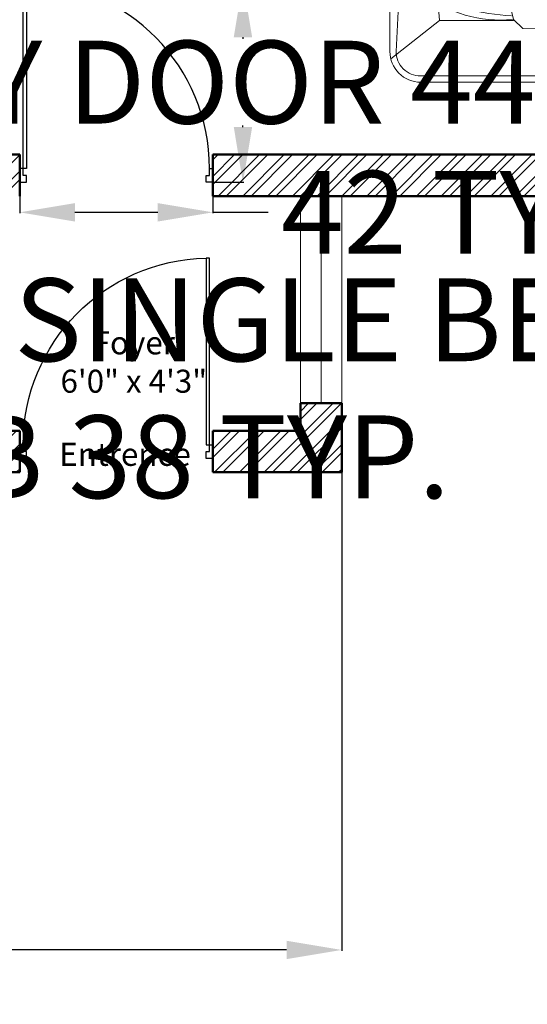
# Model space of a CAD drawing. Units: inches. Extents: x -90 to 536, y -553 to 299.
# Tile 10 of 27: x 191 to 301, y -553 to -339. Entities that reach past the tile are written whole.
import ezdxf

# ---------------------------------------------------------------- set-up
doc = ezdxf.new("R2010")
doc.units = ezdxf.units.IN
for name, color, linetype, lineweight in [('A-ANNO-DIMS', 2, 'Continuous', 18), ('A-ANNO-TEXT', 7, 'Continuous', 18), ('A-AREA-IDEN', 7, 'Continuous', 18), ('A-DOOR', 4, 'Continuous', 25), ('A-GLAZ', 4, 'Continuous', 18), ('A-WALL-PATT', 252, 'Continuous', 13), ('Furniture', 2, 'Continuous', 18), ('Outer Wall', 1, 'Continuous', 50)]:
    doc.layers.add(name, color=color, linetype=linetype, lineweight=lineweight)
doc.styles.get("Standard").update_dxf_attribs({"font": 'arial.ttf'})
doc.dimstyles.get("Standard").update_dxf_attribs({"dimtxt": 18, "dimasz": 12, "dimexe": 0.18, "dimexo": 0.0625, "dimgap": 0.09, "dimtad": 0, "dimtih": 1, "dimtoh": 1, "dimdec": 0, "dimzin": 0, "dimdsep": 46, "dimlunit": 3, "dimtxsty": 'Standard', "dimcen": 0.09, "dimadec": 0, "dimazin": 0, "dimtfac": 1, "dimtdec": 0, "dimtofl": 0, "dimtmove": 0, "dimatfit": 3, "dimfxl": 1, "dimtolj": 1, "dimtzin": 0, "dimarcsym": 0})

# ---------------------------------------------------------------- blocks, each defined once
blk = doc.blocks.new('A$C4DC51D13')
for p, q in [((3265.3, 2996.2), (1188.4, 2996.2)), ((1895.2, 2134), (1895.2, 2996.2)), ((2559.6, 2996.2), (2559.6, 2617.8)), ((277.4, 2939.6), (277.4, 2141.8)), ((943, 2103.5), (943, 2936.7)), ((1188.4, 2962.7), (1862.1, 2962.7)), ((1862.1, 2134), (1862.1, 2962.7)), ((1928.3, 2961.6), (2524.2, 2961.6)), ((1928.3, 2134), (1928.3, 2961.6)), ((2524.2, 2961.6), (2524.2, 2658.6)), ((2590.4, 2962.7), (2590.4, 2654.5)), ((3265.3, 2962.7), (2590.4, 2962.7)), ((1018.2, 2892.3), (232.2, 2892.3)), ((304, 2865.7), (304, 2253.3)), ((916.4, 2865.7), (304, 2865.7)), ((916.4, 2253.3), (916.4, 2865.7)), ((1290.4, 2664.8), (1028, 2870.9)), ((3163.3, 2664.8), (3425.7, 2870.9)), ((3778.5, 2897), (3631.2, 2747.3)), ((4008.9, 2375.5), (3778.5, 2897)), ((4156.2, 2525.2), (3778.5, 2897)), ((1022.9, 2163.8), (1022.9, 2830.3)), ((1056, 2830.3), (1081, 2194.8)), ((3397.7, 2830.3), (3364.5, 2194.8)), ((3430.8, 2163.8), (3430.8, 2830.3)), ((423.7, 2370.8), (776.6, 2723.7)), ((427.4, 2727.4), (772.8, 2367.1)), ((506.4, 2652.2), (506.4, 2704.4)), ((510.6, 2655.8), (510.6, 2706.9)), ((514.9, 2659.2), (514.9, 2709.2)), ((519.1, 2662.3), (519.1, 2711.3)), ((523.3, 2665.1), (523.3, 2713.4)), ((527.5, 2667.8), (527.5, 2715.2)), ((531.8, 2670.2), (531.8, 2717)), ((536, 2672.5), (536, 2718.7)), ((540.2, 2674.6), (540.2, 2720.2)), ((544.4, 2676.5), (544.4, 2721.6)), ((548.7, 2678.2), (548.7, 2722.9)), ((650.1, 2678.8), (650.1, 2723.3)), ((654.3, 2677.1), (654.3, 2722)), ((658.6, 2675.2), (658.6, 2720.7)), ((662.8, 2673.2), (662.8, 2719.2)), ((667, 2671), (667, 2717.6)), ((668.5, 2670.2), (668.5, 2717)), ((671.2, 2668.6), (671.2, 2715.9)), ((672.7, 2667.8), (672.7, 2715.2)), ((675.5, 2666.1), (675.5, 2714)), ((676.9, 2665.1), (676.9, 2713.4)), ((679.7, 2663.3), (679.7, 2712)), ((681.1, 2662.3), (681.1, 2711.3)), ((683.9, 2660.3), (683.9, 2709.9)), ((685.4, 2659.2), (685.4, 2709.2)), ((688.1, 2657), (688.1, 2707.7)), ((689.6, 2655.8), (689.6, 2706.9)), ((692.4, 2653.5), (692.4, 2705.3)), ((693.8, 2652.2), (693.8, 2704.4)), ((4008.9, 2375.5), (3631.2, 2747.3)), ((448.9, 2650.4), (504.4, 2650.4)), ((451.5, 2440.6), (451.5, 2654)), ((451.9, 2654.6), (509.2, 2654.6)), ((455.1, 2658.8), (514.4, 2658.8)), ((455.7, 2434.9), (455.7, 2659.6)), ((458.4, 2663.1), (520.2, 2663.1)), ((459.9, 2558.8), (459.9, 2664.9)), ((462, 2667.3), (526.7, 2667.3)), ((464.1, 2583.3), (464.1, 2669.7)), ((465.8, 2671.5), (534.1, 2671.5)), ((468.4, 2596.6), (468.4, 2674.3)), ((469.8, 2675.7), (542.8, 2675.7)), ((472.6, 2606.7), (472.6, 2678.5)), ((476.8, 2615), (476.8, 2682.5)), ((481, 2622.2), (481, 2686.2)), ((485.3, 2628.5), (485.3, 2689.7)), ((489.5, 2634.2), (489.5, 2693)), ((489.5, 2667.3), (489.5, 2633.5)), ((493.7, 2639.3), (493.7, 2696.1)), ((497.9, 2644), (497.9, 2699.1)), ((502.2, 2648.3), (502.2, 2701.8)), ((657.4, 2675.7), (730.4, 2675.7)), ((734.5, 2671.5), (666.1, 2671.5)), ((666.1, 2671.5), (734.5, 2671.5)), ((738.2, 2667.3), (673.5, 2667.3)), ((673.5, 2667.3), (738.2, 2667.3)), ((741.8, 2663.1), (680, 2663.1)), ((680, 2663.1), (741.8, 2663.1)), ((745.2, 2658.8), (685.8, 2658.8)), ((685.8, 2658.8), (745.2, 2658.8)), ((748.3, 2654.6), (691, 2654.6)), ((691, 2654.6), (748.3, 2654.6)), ((751.3, 2650.4), (695.8, 2650.4)), ((695.8, 2650.4), (751.3, 2650.4)), ((696.6, 2649.6), (696.6, 2702.7)), ((698, 2648.3), (698, 2701.8)), ((700.8, 2645.5), (700.8, 2700)), ((702.3, 2644), (702.3, 2699.1)), ((705, 2641), (705, 2697.2)), ((706.5, 2639.3), (706.5, 2696.1)), ((709.3, 2636), (709.3, 2694.1)), ((710.7, 2634.2), (710.7, 2693)), ((713.5, 2630.5), (713.5, 2690.9)), ((714.9, 2628.5), (714.9, 2689.7)), ((717.7, 2624.4), (717.7, 2687.4)), ((719.2, 2622.2), (719.2, 2686.2)), ((722, 2617.6), (722, 2683.8)), ((723.4, 2615), (723.4, 2682.5)), ((726.2, 2609.7), (726.2, 2679.9)), ((727.6, 2606.7), (727.6, 2678.5)), ((730.4, 2600.3), (730.4, 2675.7)), ((731.9, 2596.6), (731.9, 2674.3)), ((734.6, 2588.4), (734.6, 2671.3)), ((736.1, 2583.3), (736.1, 2669.7)), ((738.9, 2570.4), (738.9, 2666.6)), ((740.3, 2558.8), (740.3, 2664.9)), ((743.1, 2433.1), (743.1, 2661.5)), ((744.5, 2434.9), (744.5, 2659.6)), ((747.3, 2438.6), (747.3, 2656)), ((748.8, 2440.6), (748.8, 2654)), ((1283.3, 2574.2), (1290.4, 2664.8)), ((1290.4, 2664.8), (1894.7, 2664.8)), ((1895.2, 2663.7), (2557.3, 2663.7)), ((2603.6, 2664.8), (2559, 2664.8)), ((3163.3, 2664.8), (2764.7, 2664.8)), ((3170.4, 2574.2), (3163.3, 2664.8)), ((3631.7, 2676.6), (3938.2, 2375)), ((424.8, 2599.7), (469.6, 2599.7)), ((426.1, 2603.9), (471.3, 2603.9)), ((426.1, 2490.7), (426.1, 2603.9)), ((427.5, 2608.1), (473.3, 2608.1)), ((429.1, 2612.3), (475.4, 2612.3)), ((430.3, 2479), (430.3, 2615.5)), ((430.7, 2616.6), (477.7, 2616.6)), ((432.5, 2620.8), (480.2, 2620.8)), ((434.5, 2469.3), (434.5, 2625.2)), ((434.5, 2625), (482.9, 2625)), ((436.5, 2629.2), (485.8, 2629.2)), ((438.7, 2633.5), (488.9, 2633.5)), ((438.8, 2460.9), (438.8, 2633.6)), ((441, 2637.7), (492.3, 2637.7)), ((443, 2453.4), (443, 2641.1)), ((443.5, 2641.9), (496, 2641.9)), ((446.1, 2646.1), (500, 2646.1)), ((447.2, 2446.7), (447.2, 2647.8)), ((754.1, 2646.1), (700.2, 2646.1)), ((700.2, 2646.1), (754.1, 2646.1)), ((756.7, 2641.9), (704.2, 2641.9)), ((704.2, 2641.9), (756.7, 2641.9)), ((759.2, 2637.7), (707.9, 2637.7)), ((707.9, 2637.7), (759.2, 2637.7)), ((761.5, 2633.5), (711.3, 2633.5)), ((711.3, 2633.5), (761.5, 2633.5)), ((763.7, 2629.2), (714.4, 2629.2)), ((714.4, 2629.2), (763.7, 2629.2)), ((765.8, 2625), (717.3, 2625)), ((767.7, 2620.8), (720, 2620.8)), ((769.5, 2616.6), (722.5, 2616.6)), ((771.1, 2612.3), (724.8, 2612.3)), ((772.7, 2608.1), (726.9, 2608.1)), ((774.1, 2603.9), (728.9, 2603.9)), ((775.4, 2599.7), (730.7, 2599.7)), ((751.5, 2444.5), (751.5, 2650)), ((753, 2446.7), (753, 2647.8)), ((755.8, 2451.1), (755.8, 2643.5)), ((757.2, 2453.4), (757.2, 2641.1)), ((760, 2458.3), (760, 2636.3)), ((761.4, 2460.9), (761.4, 2633.6)), ((764.2, 2466.3), (764.2, 2628.2)), ((765.7, 2469.3), (765.7, 2625.2)), ((1798, 2530.2), (1812.1, 2637.9)), ((417.1, 2548.9), (459.4, 2548.9)), ((417.1, 2544.7), (459.5, 2544.7)), ((417.2, 2553.2), (459.6, 2553.2)), ((417.4, 2557.4), (459.8, 2557.4)), ((417.7, 2561.6), (460.2, 2561.6)), ((418.1, 2565.8), (460.7, 2565.8)), ((418.5, 2570.1), (461.3, 2570.1)), ((419.1, 2574.3), (462.1, 2574.3)), ((419.8, 2578.5), (462.9, 2578.5)), ((420.6, 2582.7), (464, 2582.7)), ((421.5, 2587), (465.2, 2587)), ((422.5, 2591.2), (466.5, 2591.2)), ((423.6, 2595.4), (467.9, 2595.4)), ((776.6, 2595.4), (732.3, 2595.4)), ((777.7, 2591.2), (733.7, 2591.2)), ((778.7, 2587), (735.1, 2587)), ((779.6, 2582.7), (736.2, 2582.7)), ((780.4, 2578.5), (737.3, 2578.5)), ((781.1, 2574.3), (738.2, 2574.3)), ((781.7, 2570.1), (738.9, 2570.1)), ((782.2, 2565.8), (739.6, 2565.8)), ((782.5, 2561.6), (740.1, 2561.6)), ((782.8, 2557.4), (740.4, 2557.4)), ((783, 2553.2), (740.7, 2553.2)), ((783.1, 2548.9), (740.8, 2548.9)), ((783.1, 2544.7), (740.8, 2544.7)), ((1022.9, 2554.4), (1249.6, 2554.4)), ((1895.5, 2582.2), (1932.3, 2494.6)), ((3430.8, 2554.4), (3204.1, 2554.4)), ((417.2, 2540.5), (459.6, 2540.5)), ((417.5, 2536.3), (459.9, 2536.3)), ((417.8, 2532), (460.3, 2532)), ((418.2, 2527.8), (460.8, 2527.8)), ((418.7, 2523.6), (461.4, 2523.6)), ((419.3, 2519.4), (462.2, 2519.4)), ((459.9, 2429.7), (459.9, 2535.7)), ((781, 2519.4), (738, 2519.4)), ((781.6, 2523.6), (738.8, 2523.6)), ((782.1, 2527.8), (739.4, 2527.8)), ((782.5, 2532), (740, 2532)), ((740.3, 2429.7), (740.3, 2535.7)), ((782.8, 2536.3), (740.4, 2536.3)), ((783, 2540.5), (740.6, 2540.5)), ((1200, 2520.5), (1251.9, 2440.8)), ((2559, 2535.8), (2557.3, 2535.8)), ((3253.7, 2520.5), (3201.8, 2440.8)), ((4008.9, 2375.5), (4156.2, 2525.2)), ((1243.2, 2146.7), (1272.2, 2431.8)), ((3210.5, 2146.7), (3181.5, 2431.8)), ((242.9, 2226.7), (1018.2, 2226.7)), ((304, 2253.3), (916.4, 2253.3)), ((1081, 2194.8), (1243.2, 2146.7)), ((3364.5, 2194.8), (3210.5, 2146.7)), ((498.8, 1837.1), (382.1, 2139.5)), ((1040.3, 1942.9), (421.2, 2132.6)), ((1145.1, 2159.3), (1022.9, 2163.8)), ((1145.1, 2159.3), (1243.2, 2146.7)), ((1244.8, 2113), (1243.2, 2146.7)), ((2590.4, 2164.3), (2590.4, 2134)), ((3208.9, 2113), (3210.5, 2146.7)), ((3308.6, 2159.3), (3210.5, 2146.7)), ((3308.6, 2159.3), (3430.8, 2163.8)), ((411.8, 2101.9), (992.6, 1890.2)), ((1839.5, 2113), (1244.8, 2113)), ((1839.5, 2079.9), (1244.8, 2079.9)), ((2308.5, 2111.9), (1950.4, 2111.9)), ((2322.1, 2078.8), (1950.4, 2078.8)), ((2614.2, 2113), (3208.9, 2113)), ((2614.2, 2079.9), (3208.9, 2079.9)), ((220.3, 2026), (19.3, 1370.1)), ((251.1, 2016.6), (37.1, 1314.7)), ((677.4, 2054.1), (612.9, 1843.6)), ((1009.7, 1828.1), (1040.3, 1942.9)), ((658.5, 1880), (717.8, 1809.1)), ((992.6, 1890.2), (993.4, 1733.4)), ((1158.3, 1784.3), (1158.3, 1858.2)), ((1181.8, 1784.3), (1181.8, 1858.2)), ((1205.3, 1784.3), (1205.3, 1858.2)), ((1228.8, 1784.3), (1228.8, 1858.2)), ((1252.2, 1784.3), (1252.2, 1858.2)), ((1319.4, 1784.3), (1319.4, 1858.2)), ((1342.9, 1784.3), (1342.9, 1858.2)), ((1366.3, 1784.3), (1366.3, 1858.2)), ((1389.8, 1784.3), (1389.8, 1858.2)), ((1413.3, 1784.3), (1413.3, 1858.2)), ((1436.8, 1784.3), (1436.8, 1858.2)), ((1460.2, 1784.3), (1460.2, 1858.2)), ((1483.7, 1784.3), (1483.7, 1858.2)), ((1507.2, 1784.3), (1507.2, 1858.2)), ((1530.7, 1784.3), (1530.7, 1858.2)), ((1554.1, 1784.3), (1554.1, 1858.2)), ((1577.6, 1784.3), (1577.6, 1858.2)), ((1714.2, 1784.3), (1714.2, 1858.2)), ((1737.6, 1784.3), (1737.6, 1858.2)), ((1761.1, 1784.3), (1761.1, 1858.2)), ((1784.6, 1784.3), (1784.6, 1858.2)), ((1808.1, 1784.3), (1808.1, 1858.2)), ((1831.5, 1784.3), (1831.5, 1858.2)), ((1855, 1784.3), (1855, 1858.2)), ((1878.5, 1784.3), (1878.5, 1858.2)), ((1902, 1784.3), (1902, 1858.2)), ((2050.7, 1784.3), (2050.7, 1858.2)), ((2074.2, 1784.3), (2074.2, 1858.2)), ((2097.7, 1784.3), (2097.7, 1858.2)), ((2121.1, 1784.3), (2121.1, 1858.2)), ((2144.6, 1784.3), (2144.6, 1858.2)), ((2168.1, 1784.3), (2168.1, 1858.2)), ((2191.6, 1782.4), (2191.6, 1856.3)), ((2238.5, 1785.1), (2238.5, 1859)), ((2262, 1784.3), (2262, 1858.2)), ((2285.4, 1784.3), (2285.4, 1858.2)), ((2543.7, 1784.3), (2543.7, 1858.2)), ((2567.1, 1784.3), (2567.1, 1858.2)), ((2590.6, 1784.3), (2590.6, 1858.2)), ((2614.1, 1784.3), (2614.1, 1858.2)), ((2661, 1784.3), (2661, 1858.2)), ((2684.5, 1784.3), (2684.5, 1858.2)), ((2708, 1772.3), (2708, 1858.2)), ((2731.5, 1784.3), (2731.5, 1858.2)), ((2754.9, 1784.3), (2754.9, 1858.2)), ((2778.4, 1784.3), (2778.4, 1858.2)), ((2801.9, 1784.3), (2801.9, 1858.2)), ((2825.4, 1784.3), (2825.4, 1858.2)), ((2848.8, 1784.3), (2848.8, 1858.2)), ((2872.3, 1784.3), (2872.3, 1858.2)), ((2895.8, 1784.3), (2895.8, 1858.2)), ((2919.3, 1784.3), (2919.3, 1858.2)), ((2942.7, 1784.3), (2942.7, 1858.2)), ((2966.2, 1744.8), (2966.2, 1858.2)), ((2989.7, 1784.3), (2989.7, 1858.2)), ((3013.2, 1772.3), (3013.2, 1858.2)), ((3036.6, 1784.3), (3036.6, 1858.2)), ((3060.1, 1784.3), (3060.1, 1858.2)), ((3083.6, 1784.3), (3083.6, 1858.2)), ((498.8, 1837.1), (341.4, 1323.6)), ((584.9, 1817.9), (498.8, 1837.1)), ((1009.7, 1828.1), (993.4, 1733.4)), ((1158.3, 1821.3), (1158.5, 487.7)), ((2215, 1785.7), (2215, 1832.3)), ((993.4, 1733.4), (720.4, 1787.6)), ((1162.1, 1754.9), (1088.2, 1754.9)), ((1166.1, 1769.7), (1091.8, 1794.5)), ((3248.4, 1772.3), (1158.5, 1772.3)), ((3248.4, 487.7), (3248.4, 1772.3)), ((3248.8, 1760.8), (3322.7, 1760.8)), ((1024.2, 1722.3), (842.3, 1125.2)), ((873.1, 1115.8), (1055, 1712.9)), ((1024.2, 1722.3), (993.4, 1733.4)), ((1162.1, 1741.1), (1088.2, 1741.1)), ((1162.1, 1717.6), (1088.2, 1717.6)), ((1162.1, 1708), (1088.2, 1708)), ((1196, 511), (1196, 1744.8)), ((1196, 1744.8), (3215.6, 1744.8)), ((3215.6, 511), (3215.6, 1744.8)), ((3248.8, 1737.3), (3322.7, 1737.3)), ((3248.8, 1713.8), (3322.7, 1713.8)), ((3600.6, 1621.7), (3605.1, 1743.8)), ((3605.1, 1743.8), (4271.6, 1743.8)), ((4271.6, 1710.7), (3636.1, 1685.8)), ((3995.7, 1743.8), (3995.7, 1517.1)), ((4106.1, 1476.4), (4312.2, 1738.8)), ((1162.1, 1684.5), (1088.2, 1684.5)), ((3248.8, 1690.4), (3322.7, 1690.4)), ((3248.8, 1666.9), (3322.7, 1666.9)), ((3248.8, 1643.4), (3322.7, 1643.4)), ((3636.1, 1685.8), (3588, 1523.6)), ((3248.8, 1619.9), (3322.7, 1619.9)), ((3600.6, 1621.7), (3588, 1523.6)), ((4404, 1578.3), (4404, 904.6)), ((4437.5, 165.9), (4437.5, 1578.3)), ((1162.1, 1492.9), (1088.2, 1492.9)), ((1701.7, 1530), (1701.7, 911.2)), ((2593.1, 907.9), (2593.1, 1490.3)), ((2629.1, 907.9), (2629.1, 1503.1)), ((3248.8, 1513.8), (3322.7, 1513.8)), ((3248.8, 1513.3), (3322.7, 1513.3)), ((3248.8, 1490.4), (3322.7, 1490.4)), ((3248.8, 1489.9), (3322.7, 1489.9)), ((3521.2, 1130.7), (3521.2, 1521.9)), ((3554.3, 1131.4), (3554.3, 1521.9)), ((3588, 1523.6), (3873.1, 1494.5)), ((1162.1, 1483.3), (1088.2, 1483.3)), ((1162.1, 1459.8), (1088.2, 1459.8)), ((1162.1, 1446), (1088.2, 1446)), ((2674.6, 1449.9), (1641, 1449.9)), ((1888.1, 1449.9), (1701.7, 1263.5)), ((1856.2, 1449.9), (1701.7, 1295.4)), ((1715.1, 1449.9), (1701.7, 1436.5)), ((1737.7, 1483.1), (1737.7, 911.2)), ((2343.3, 1449.9), (1855.3, 961.9)), ((2629.1, 1449), (2142, 961.9)), ((2325.1, 1449.9), (2154.2, 1279.1)), ((2461.6, 1449.9), (2177, 1165.3)), ((3248.8, 1466.9), (3322.7, 1466.9)), ((3248.8, 1443.4), (3322.7, 1443.4)), ((4015.5, 1483.4), (4106.1, 1476.4)), ((4106.1, 1476.4), (4106.1, 872.1)), ((1162.1, 1412.8), (1088.2, 1412.8)), ((1162.1, 1399), (1088.2, 1399)), ((2674.6, 1413.9), (1641, 1413.9)), ((3248.8, 1419.9), (3322.7, 1419.9)), ((3250, 1407.8), (3519, 1407.8)), ((6.3, 1324.2), (19.3, 1370.2)), ((479.3, 1327.3), (375.2, 1344.9)), ((1162.1, 1375.5), (1088.2, 1375.5)), ((1162.1, 1352.1), (1088.2, 1352.1)), ((1162.1, 1342.9), (1088.2, 1342.9)), ((1162.1, 1342.4), (1088.2, 1342.4)), ((3248.8, 990.8), (3248.4, 1328.4)), ((3248.8, 1359), (3322.7, 1359)), ((342.8, 1324.6), (76.7, 1139.6)), ((843, 1127.6), (342.8, 1324.6)), ((369.2, 1044.8), (442.9, 1285.2)), ((1162.1, 1319.4), (1088.2, 1319.4)), ((1162.1, 1318.9), (1088.2, 1318.9)), ((1162.1, 1296), (1088.2, 1296)), ((1162.1, 1295.5), (1088.2, 1295.5)), ((1196, 1272.5), (1088.2, 1272.5)), ((2629.1, 1280.5), (2310.5, 961.9)), ((3248.8, 1312.1), (3322.7, 1312.1)), ((3248.8, 1302.3), (3322.7, 1302.3)), ((3250, 1317.8), (3519, 1317.8)), ((1162.1, 1272), (1088.2, 1272)), ((1162.1, 1249), (1088.2, 1249)), ((1162.1, 1248.5), (1088.2, 1248.5)), ((1162.1, 1225.5), (1088.2, 1225.5)), ((3248.8, 1249), (3322.7, 1249)), ((3248.8, 1248.5), (3322.7, 1248.5)), ((3248.8, 1239.3), (3322.7, 1239.3)), ((3248.8, 1238.8), (3322.7, 1238.8)), ((3248.8, 1225.5), (3322.7, 1225.5)), ((1162.1, 1202.1), (1088.2, 1202.1)), ((1196, 1178.6), (1088.2, 1178.6)), ((3248.8, 1202.1), (3322.7, 1202.1)), ((3248.8, 1178.6), (3322.7, 1178.6)), ((732, 933.5), (112.9, 1123.3)), ((122.4, 1154.1), (719.7, 996.3)), ((719.7, 996.3), (810.6, 1133.2)), ((771, 1045.7), (810.6, 1133.2)), ((842.3, 1125.2), (810.6, 1133.2)), ((1162.1, 1155.1), (1088.2, 1155.1)), ((1162.1, 1131.6), (1088.2, 1131.6)), ((1728.6, 1158.4), (1701.7, 1131.5)), ((3248.8, 1155.1), (3322.7, 1155.1)), ((3248.8, 1131.6), (3322.7, 1131.6)), ((1162.1, 1108.2), (1088.2, 1108.2)), ((1162.1, 1084.7), (1088.2, 1084.7)), ((1196, 1061.2), (1088.2, 1061.2)), ((3248.8, 1108.2), (3322.7, 1108.2)), ((771, 1045.7), (732, 933.5)), ((1162.1, 1037.7), (1088.2, 1037.7)), ((1162.1, 1014.3), (1088.2, 1014.3)), ((1648.3, 1019.6), (2616.7, 1019.6)), ((1926.6, 1051.5), (1837.1, 961.9)), ((2629.1, 1012), (2579, 961.9)), ((3248.8, 1014.3), (3322.7, 1014.3)), ((1196, 967.3), (1088.2, 967.3)), ((1648.3, 961.9), (2681.9, 961.9)), ((2006.3, 994.6), (1973.6, 961.9)), ((2459.2, 974.1), (2447, 961.9)), ((3248.8, 990.8), (3322.7, 990.8)), ((3248.8, 967.3), (3322.7, 967.3)), ((1162.1, 943.8), (1088.2, 943.8)), ((1162.1, 920.4), (1088.2, 920.4)), ((3248.8, 943.8), (3322.7, 943.8)), ((3248.8, 920.4), (3322.7, 920.4)), ((4097.4, 904.6), (4404, 904.6)), ((1196, 860.5), (1088.2, 860.5)), ((4106.1, 871.5), (4437.5, 871.5)), ((1162.1, 837), (1088.2, 837)), ((1162.1, 813.5), (1088.2, 813.5)), ((3521.2, 816.9), (3521.2, 222.3)), ((3554.3, 816.9), (3554.3, 222.3)), ((4404, 840.7), (4110.5, 840.7)), ((4404, 165.9), (4404, 840.7)), ((1162.1, 790), (1031.8, 790)), ((1196, 766.6), (1088.2, 766.6)), ((1162.1, 743.1), (1088.2, 743.1)), ((1162.1, 719.6), (1088.2, 719.6)), ((4106.1, 267.8), (4106.1, 666.5)), ((1162.1, 627.8), (1088.2, 627.8)), ((1162.1, 604.4), (1088.2, 604.4)), ((3248.8, 627.8), (3322.7, 627.8)), ((3248.8, 604.4), (3322.7, 604.4)), ((1162.1, 580.9), (1034.2, 580.9)), ((1162.1, 557.4), (1088.2, 557.4)), ((1162.1, 533.9), (1088.2, 533.9)), ((3248.8, 580.9), (3322.7, 580.9)), ((3248.8, 557.4), (3322.7, 557.4)), ((3248.8, 533.9), (3322.7, 533.9)), ((1162.1, 510.5), (1088.2, 510.5)), ((1162, 495.1), (1116.6, 429)), ((1158.5, 487.7), (3248.4, 487.7)), ((3215.6, 511), (1196, 511)), ((1311.1, 487.7), (1311.1, 402.4)), ((1334.6, 511), (1334.6, 402.4)), ((1381.6, 511), (1381.6, 402.4)), ((1428.5, 487.7), (1428.5, 402.4)), ((1498.9, 487.7), (1498.9, 402.4)), ((1522.4, 487.7), (1522.4, 402.4)), ((1663.3, 487.7), (1663.3, 402.4)), ((1757.8, 487.7), (1757.8, 402.4)), ((1781.3, 487.7), (1781.3, 402.4)), ((1922.1, 487.7), (1922.1, 402.4)), ((2036, 487.7), (2036, 402.4)), ((2059.5, 511), (2059.5, 402.4)), ((2106.4, 511), (2106.4, 402.4)), ((2153.4, 487.7), (2153.4, 402.4)), ((2223.8, 487.7), (2223.8, 402.4)), ((2247.2, 487.7), (2247.2, 402.4)), ((2388.1, 487.7), (2388.1, 402.4)), ((2482, 487.7), (2482, 402.4)), ((2505.5, 487.7), (2505.5, 402.4)), ((2669.8, 511), (2669.8, 402.4)), ((2740.2, 487.7), (2740.2, 402.4)), ((2784.9, 487.7), (2784.9, 402.4)), ((2904.5, 487.7), (2904.5, 402.4)), ((3021.9, 487.7), (3021.9, 402.4)), ((3092.7, 484.5), (3092.7, 410.6)), ((3116.2, 484.5), (3116.2, 410.6)), ((3244.9, 495.1), (3290.3, 429)), ((3248.8, 510.5), (3322.7, 510.5)), ((1167.1, 476.3), (1167.1, 402.4)), ((1190.6, 476.3), (1190.6, 402.4)), ((1214, 476.3), (1214, 402.4)), ((1237.5, 476.3), (1237.5, 402.4)), ((1358.1, 476.3), (1358.1, 402.4)), ((1405, 476.3), (1405, 402.4)), ((1452, 476.3), (1452, 402.4)), ((1475.5, 476.3), (1475.5, 402.4)), ((1545.9, 476.3), (1545.9, 402.4)), ((1569.4, 476.3), (1569.4, 402.4)), ((1592.8, 476.3), (1592.8, 402.4)), ((1616.3, 476.3), (1616.3, 402.4)), ((1639.8, 476.3), (1639.8, 402.4)), ((1804.8, 476.3), (1804.8, 402.4)), ((1828.2, 476.3), (1828.2, 402.4)), ((1851.7, 476.3), (1851.7, 402.4)), ((1875.2, 476.3), (1875.2, 402.4)), ((1898.7, 476.3), (1898.7, 402.4)), ((2082.9, 476.3), (2082.9, 402.4)), ((2129.9, 476.3), (2129.9, 402.4)), ((2176.8, 476.3), (2176.8, 402.4)), ((2200.3, 476.3), (2200.3, 402.4)), ((2270.7, 476.3), (2270.7, 402.4)), ((2294.2, 476.3), (2294.2, 402.4)), ((2317.7, 476.3), (2317.7, 402.4)), ((2341.1, 476.3), (2341.1, 402.4)), ((2364.6, 476.3), (2364.6, 402.4)), ((2411.6, 476.3), (2411.6, 402.4)), ((2435, 476.3), (2435, 402.4)), ((2458.5, 476.3), (2458.5, 402.4)), ((2528.9, 476.3), (2528.9, 402.4)), ((2552.4, 476.3), (2552.4, 402.4)), ((2575.9, 476.3), (2575.9, 402.4)), ((2599.4, 476.3), (2599.4, 402.4)), ((2622.8, 476.3), (2622.8, 402.4)), ((2646.3, 476.3), (2646.3, 402.4)), ((2693.3, 476.3), (2693.3, 402.4)), ((2716.7, 476.3), (2716.7, 402.4)), ((2738, 476.3), (2738, 402.4)), ((2761.5, 476.3), (2761.5, 402.4)), ((2763.7, 476.3), (2763.7, 402.4)), ((2787.2, 476.3), (2787.2, 402.4)), ((2808.4, 476.3), (2808.4, 402.4)), ((2810.6, 476.3), (2810.6, 402.4)), ((2831.9, 476.3), (2831.9, 402.4)), ((2834.1, 476.3), (2834.1, 402.4)), ((2855.4, 476.3), (2855.4, 402.4)), ((2857.6, 476.3), (2857.6, 402.4)), ((2878.8, 476.3), (2878.8, 402.4)), ((2881.1, 476.3), (2881.1, 402.4)), ((2902.3, 476.3), (2902.3, 402.4)), ((2925.8, 476.3), (2925.8, 402.4)), ((2928, 476.3), (2928, 402.4)), ((2949.3, 476.3), (2949.3, 402.4)), ((2951.5, 476.3), (2951.5, 402.4)), ((2972.7, 476.3), (2972.7, 402.4)), ((2975, 476.3), (2975, 402.4)), ((2996.2, 476.3), (2996.2, 402.4)), ((2998.4, 476.3), (2998.4, 402.4)), ((3019.7, 476.3), (3019.7, 402.4)), ((3043.2, 476.3), (3043.2, 402.4)), ((3045.4, 476.3), (3045.4, 402.4)), ((3066.6, 476.3), (3066.6, 402.4)), ((3068.9, 476.3), (3068.9, 402.4)), ((3092.3, 476.3), (3092.3, 402.4)), ((3115.8, 476.3), (3115.8, 402.4)), ((3202.2, 476.3), (3202.2, 402.4)), ((3225.7, 476.3), (3225.7, 402.4)), ((3249.2, 476.3), (3249.2, 402.4)), ((4015.5, 260.8), (4106.1, 267.8)), ((4106.1, 267.8), (4312.2, 5.4)), ((3588, 220.6), (3873.1, 249.7)), ((3636.1, 66.6), (3588, 220.6)), ((3961.8, 177.4), (3882.1, 229.3)), ((3995.7, 0.4), (3995.7, 227)), ((3600.6, 122.5), (3605.1, 0.4)), ((4271.6, 33.5), (3636.1, 66.6)), ((3605.1, 0.4), (4271.6, 0.4))]:
    blk.add_line(p, q)
at = {"linetype": 'ByBlock'}
for points in [[(2342.9, 1843.9), (2352.5, 1810.4), (2340.1, 1777.7), (2351.8, 1757), (2412.3, 1818), (2433.1, 1866.4), (2453.1, 1889.5), (2436, 1914.7), (2407.6, 1926.2), (2433.7, 1959.9), (2473.1, 2048.3), (2530.6, 2101.1), (2625.9, 2180.3), (2669, 2174.2), (2748.1, 2315.4), (2745.8, 2342.6), (2801.2, 2404.9), (2823.9, 2479.6), (2818.4, 2529.9), (2775.1, 2571.7), (2782.4, 2583.3), (2765.2, 2658.8), (2714.5, 2706.9), (2634.6, 2708.6), (2571.9, 2652.6), (2548.8, 2649.4), (2474, 2672.1), (2312.9, 2542.1), (2312.9, 2341.6), (2333.9, 2336.4), (2302, 2223.9), (2313.6, 2216.6), (2297.4, 2095.7), (2309.3, 2034.9), (2320.2, 1952), (2319.3, 1929.9), (2280.8, 1863.6), (2257.7, 1842.4), (2239.2, 1825.7), (2220.1, 1798.2), (2221.6, 1713.1), (2254.3, 1700.7), (2275.9, 1729.8), (2288.6, 1768), (2313.7, 1797.6)], [(3285.2, 1088.3), (3251.7, 1078.6), (3219, 1091.1), (3198.3, 1079.4), (3259.3, 1018.8), (3307.7, 998), (3330.8, 978), (3356, 995.1), (3367.5, 1023.6), (3401.2, 997.5), (3489.6, 958), (3542.4, 900.5), (3621.6, 805.3), (3615.5, 762.2), (3756.7, 683), (3783.9, 685.3), (3846.2, 629.9), (3920.9, 607.2), (3971.2, 612.7), (4013, 656), (4024.6, 648.7), (4100.1, 665.9), (4148.2, 716.6), (4149.9, 796.5), (4093.9, 859.3), (4090.7, 882.4), (4113.4, 957.1), (3983.4, 1118.2), (3782.9, 1118.2), (3777.7, 1097.2), (3665.2, 1129.2), (3657.9, 1117.6), (3537, 1133.7), (3476.2, 1121.9), (3393.3, 1110.9), (3371.2, 1111.9), (3304.9, 1150.4), (3283.7, 1173.4), (3267, 1191.9), (3239.5, 1211), (3154.4, 1209.5), (3142, 1176.8), (3171.1, 1155.3), (3209.3, 1142.5), (3238.9, 1117.5)]]:
    blk.add_lwpolyline(points, close=True, dxfattribs=at)
for points in [[(2563.4, 2654.7), (2512.2, 2609.3), (2506.2, 2548.3), (2540.1, 2504.4), (2576.9, 2490.9), (2579.8, 2539.3), (2598.7, 2543.6), (2636.7, 2516.4), (2690.3, 2516.7), (2731.2, 2520.1), (2758.5, 2540.1), (2773, 2563.3)], [(2629.1, 2357.8), (2507, 2405.5), (2433.2, 2450.3), (2445.5, 2500.8), (2478.9, 2546.1), (2402.4, 2506.9), (2373.4, 2424.8), (2384.4, 2341.9), (2352.8, 2340.7)], [(2712.3, 2515.8), (2652.7, 2472.4), (2603.2, 2489), (2580, 2503.6)], [(2433.2, 2450.3), (2377.6, 2423.8)], [(2738, 2438.2), (2699.2, 2425.4), (2742.4, 2401.4), (2680.4, 2403.2), (2604.1, 2328.3), (2519.2, 2273.3), (2529.8, 2261.8), (2402.7, 2252.7), (2395.4, 2241.1), (2431.1, 2241.3), (2375.7, 2196.9), (2385.2, 2181.2), (2474.4, 2199.5), (2549.9, 2234.6), (2596.2, 2223.2), (2730.1, 2333.1)], [(2374.9, 2339.8), (2395.2, 2276.9)], [(2409.5, 2153), (2387.5, 2153.9), (2359, 2165.4), (2352.6, 2193.7), (2353.5, 2215.7), (2330.5, 2194.6), (2322.1, 2196.7), (2341.8, 2240.9), (2345.5, 2329.1)], [(2431.4, 2187.8), (2379.5, 2066.7), (2320.2, 1929.7)], [(2613.2, 2183.4), (2541.6, 2218.8)], [(2407.6, 1926.2), (2342.9, 1843.9)], [(2412.9, 1911.5), (2401.6, 1865.2), (2361.9, 1812.5)], [(2279.2, 1765.9), (2259.2, 1757.4), (2247.6, 1764.7), (2246.4, 1796.2), (2253.5, 1843.5)], [(3207.2, 1152), (3198.7, 1171.9), (3206, 1183.5), (3237.5, 1184.7), (3284.8, 1177.6)], [(3352.8, 1018.2), (3306.5, 1029.5), (3253.8, 1069.2)], [(3367.5, 1023.6), (3285.2, 1088.3)], [(3629.1, 999.7), (3508, 1051.6), (3371, 1110.9)], [(3594.3, 1021.6), (3595.2, 1043.7), (3606.7, 1072.1), (3635, 1078.6), (3657, 1077.6), (3635.9, 1100.6), (3638, 1109.1), (3682.2, 1089.3), (3770.4, 1085.6)], [(3799.1, 802), (3846.8, 924.2), (3891.6, 998), (3942.1, 985.6), (3987.4, 952.2), (3948.2, 1028.7), (3866.1, 1057.7), (3783.2, 1046.8), (3782, 1078.3)], [(3879.5, 693.2), (3866.7, 732), (3842.7, 688.8), (3844.5, 750.8), (3769.6, 827.1), (3714.6, 911.9), (3703.1, 901.3), (3694, 1028.4), (3682.4, 1035.7), (3682.6, 1000), (3638.2, 1055.5), (3622.5, 1045.9), (3640.8, 956.7), (3675.9, 881.2), (3664.5, 834.9), (3774.4, 701)], [(3781.1, 1056.2), (3718.2, 1035.9)], [(3891.6, 998), (3865.1, 1053.5)], [(4096, 867.7), (4050.6, 918.9), (3989.6, 924.9), (3945.7, 891.1), (3932.2, 854.2), (3980.6, 851.3), (3984.9, 832.4), (3957.7, 794.4), (3958, 740.9), (3961.4, 699.9), (3981.4, 672.7), (4004.6, 658.1)], [(3624.7, 817.9), (3660.1, 889.6)], [(3957.1, 718.8), (3913.7, 778.5), (3930.3, 827.9), (3944.9, 851.1)]]:
    blk.add_lwpolyline(points, dxfattribs=at)
for centre, radius in [((600.1, 2547.3), 183), ((600.1, 2547.3), 140.7), ((1803.2, 1372.6), 25.7), ((2527.6, 1372.6), 25.7), ((1803.2, 1039.3), 25.7), ((2527.6, 1039.3), 25.7), ((2817.9, 923.4), 31.7), ((2095.7, 858), 41)]:
    blk.add_circle(centre, radius)
for centre, radius, start, end in [((1188.4, 2830.3), 165.9, 90, 180), ((3265.3, 2830.3), 165.9, 0, 90), ((1188.4, 2830.3), 132.4, 90, 180), ((3265.3, 2830.3), 132.4, 0, 90), ((3666.8, 2712.2), 50, 135.4503, 225.4503), ((1626.8, 1949.8), 712.7, 74.928, 126.7929), ((2192.2, 2032.6), 624.6, 69.4145, 118.3621), ((2633.9, 373.6), 2292.5, 91.8726, 91.9144), ((2832.8, 1963.1), 698.5, 52.9389, 95.0789), ((1707.9, 1527), 1115.8, 84.6406, 117.0804), ((2210.2, 1780.8), 852.5, 76.866, 111.6839), ((2713.3, 1357.7), 1282.3, 65.0725, 87.2152), ((1459.9, 2882.7), 488.4, 244.7866, 313.8058), ((2216, 2892.1), 488.4, 234.4888, 282.1285), ((2993.8, 2882.7), 488.4, 248.2152, 295.2134), ((3973.2, 2410.6), 50, 225.4503, 315.4503), ((374.1, 1978.9), 160.8, 72.9571, 162.9571), ((1234.5, 2169.3), 90, 186.4251, 276.5821), ((1839.5, 2135.1), 22.1, 270, 0), ((1839.5, 2135.1), 55.2, 270, 0), ((1950.4, 2134), 55.2, 180, 270), ((1950.4, 2134), 22.1, 180, 270), ((2619.6, 2148.3), 68.5, 191.0595, 265.4426), ((2614.2, 2135.1), 22.1, 180, 270), ((3219.2, 2169.3), 90, 263.4179, 353.5749), ((374.1, 1978.9), 128.6, 72.9571, 162.9571), ((1584.7, 1047), 1245.7, 138.0296, 166.1636), ((1067.1, 1321), 692.3, 126.1642, 178.0291), ((248.2, 1741.7), 474.4, 299.1514, 8.1705), ((974.8, 1747.9), 87.4, 336.375, 66.532), ((4271.6, 1578.3), 165.9, 0, 90), ((4271.6, 1578.3), 132.4, 0, 90), ((944.2, 1233.8), 467.1, 309.4804, 56.621), ((3610.6, 1532.2), 90, 96.4251, 186.5821), ((3383, 1136.2), 721.4, 348.1046, 36.6442), ((2968.3, 1058.8), 1115.8, 356.7543, 27.0804), ((4324, 1306.8), 488.4, 154.7866, 202.7137), ((160.1, 1277), 160.8, 162.9571, 252.9571), ((160.1, 1277), 128.6, 162.9571, 252.9571), ((2517.5, 1143.6), 586.7, 287.3395, 13.1463), ((787.1, 1131.7), 87.4, 259.3822, 349.5393), ((2356.9, 1798.1), 1287.8, 212.1153, 261.9323), ((-29968.2, -49615.7), 59944, 56.743614, 57.623407), ((3404.4, 598.4), 698.5, 322.9389, 5.0789), ((2799, 717.9), 1282.3, 335.0725, 357.2152), ((2591.9, -2109.1), 2694.5, 80.9842, 100.0261), ((4324, 437.4), 488.4, 158.2152, 205.2134), ((3610.6, 212), 90, 173.4179, 263.5749), ((4271.6, 165.9), 132.4, 270, 0), ((4271.6, 165.9), 165.9, 270, 0)]:
    blk.add_arc(centre, radius, start, end)
blk = doc.blocks.new('DOOR-42')
for points in [[(0.75, 3), (0.75, 43.5), (1.5, 43.5), (1.5, 3)], [(0, 0), (1.5, 0), (1.5, 1.5), (0.75, 1.5), (0.75, 3), (0, 3)], [(42, 0), (40.5, 0), (40.5, 1.5), (41.25, 1.5), (41.25, 3), (42, 3)]]:
    blk.add_lwpolyline(points, close=True)
blk.add_arc((0.74, 3), 40.51, 0, 88.9291)
blk = doc.blocks.new('*D27')
at = {"layer": 'A-ANNO-DIMS', "color": 0, "lineweight": -2, "transparency": 16777216}
for p, q in [((49.13, -428.62), (49.13, -434.36)), ((86.63, -428.62), (86.63, -434.36)), ((61.13, -434.18), (74.63, -434.18)), ((86.63, -434.18), (98.63, -434.18))]:
    blk.add_line(p, q, dxfattribs=at)
at = {"layer": 'A-ANNO-DIMS', "color": 0, "transparency": 16777216}
for points in [[(61.13, -432.18), (61.13, -436.18), (49.13, -434.18)], [(74.63, -432.18), (74.63, -436.18), (86.63, -434.18)]]:
    blk.add_solid(points, dxfattribs=at)
at = {"layer": 'Defpoints', "color": 0, "transparency": 16777216}
for p in [(49.13, -428.55), (86.63, -428.55), (86.63, -434.18)]:
    blk.add_point(p, dxfattribs=at)
at = {"layer": 'A-ANNO-DIMS', "color": 0, "transparency": 16777216, "insert": (195.17, -434.18), "char_height": 18, "attachment_point": 5}
blk.add_mtext('\\A1;DOOR B 38 TYP.', dxfattribs=at)
blk = doc.blocks.new('*D35')
at = {"layer": 'A-ANNO-DIMS', "color": 0, "lineweight": -2, "transparency": 16777216}
for p, q in [((233.19, -331.05), (239.84, -331.05)), ((239.66, -343.05), (239.66, -343.4)), ((239.66, -362.55), (239.66, -362.21)), ((233.19, -374.55), (239.84, -374.55))]:
    blk.add_line(p, q, dxfattribs=at)
at = {"layer": 'A-ANNO-DIMS', "color": 0, "transparency": 16777216}
for points in [[(237.66, -343.05), (241.66, -343.05), (239.66, -331.05)], [(237.66, -362.55), (241.66, -362.55), (239.66, -374.55)]]:
    blk.add_solid(points, dxfattribs=at)
at = {"layer": 'Defpoints', "color": 0, "transparency": 16777216}
for p in [(233.13, -331.05), (239.66, -331.05), (233.13, -374.55)]:
    blk.add_point(p, dxfattribs=at)
at = {"layer": 'A-ANNO-DIMS', "color": 0, "transparency": 16777216, "insert": (239.66, -352.8), "char_height": 18, "attachment_point": 5}
blk.add_mtext('\\A1;ENTRY DOOR 44 TYP.', dxfattribs=at)
blk = doc.blocks.new('*D36')
at = {"layer": 'A-ANNO-DIMS', "color": 0, "lineweight": -2, "transparency": 16777216}
for p, q in [((191.13, -374.62), (191.13, -381.26)), ((233.13, -374.62), (233.13, -381.26)), ((203.13, -381.08), (221.13, -381.08)), ((233.13, -381.08), (245.13, -381.08))]:
    blk.add_line(p, q, dxfattribs=at)
at = {"layer": 'A-ANNO-DIMS', "color": 0, "transparency": 16777216}
for points in [[(203.13, -379.08), (203.13, -383.08), (191.13, -381.08)], [(221.13, -379.08), (221.13, -383.08), (233.13, -381.08)]]:
    blk.add_solid(points, dxfattribs=at)
at = {"layer": 'Defpoints', "color": 0, "transparency": 16777216}
for p in [(191.13, -374.55), (233.13, -374.55), (233.13, -381.08)]:
    blk.add_point(p, dxfattribs=at)
at = {"layer": 'A-ANNO-DIMS', "color": 0, "transparency": 16777216, "insert": (289.39, -381.08), "char_height": 18, "attachment_point": 5}
blk.add_mtext('\\A1;42 TYP.', dxfattribs=at)
blk = doc.blocks.new('*D51')
at = {"layer": 'A-ANNO-DIMS', "color": 0, "lineweight": -2, "transparency": 16777216}
for p, q in [((96.81, -393.34), (96.81, -404.61)), ((171.13, -393.34), (171.13, -404.61)), ((108.81, -404.43), (159.13, -404.43)), ((171.13, -404.43), (183.13, -404.43))]:
    blk.add_line(p, q, dxfattribs=at)
at = {"layer": 'A-ANNO-DIMS', "color": 0, "transparency": 16777216}
for points in [[(108.81, -402.43), (108.81, -406.43), (96.81, -404.43)], [(159.13, -402.43), (159.13, -406.43), (171.13, -404.43)]]:
    blk.add_solid(points, dxfattribs=at)
at = {"layer": 'Defpoints', "color": 0, "transparency": 16777216}
for p in [(96.81, -393.28), (171.13, -393.28), (171.13, -404.43)]:
    blk.add_point(p, dxfattribs=at)
at = {"layer": 'A-ANNO-DIMS', "color": 0, "transparency": 16777216, "insert": (274.99, -404.43), "char_height": 18, "attachment_point": 5}
blk.add_mtext('\\A1;SINGLE BED 74', dxfattribs=at)
blk = doc.blocks.new('*D67')
at = {"layer": 'A-ANNO-DIMS', "color": 0, "lineweight": -2, "transparency": 16777216}
for p, q in [((261.13, -437.62), (261.13, -541.49)), ((38.13, -503.62), (38.13, -541.49)), ((50.13, -541.31), (129.5, -541.31)), ((249.13, -541.31), (169.76, -541.31))]:
    blk.add_line(p, q, dxfattribs=at)
at = {"layer": 'A-ANNO-DIMS', "color": 0, "transparency": 16777216}
for points in [[(50.13, -539.31), (50.13, -543.31), (38.13, -541.31)], [(249.13, -539.31), (249.13, -543.31), (261.13, -541.31)]]:
    blk.add_solid(points, dxfattribs=at)
at = {"layer": 'Defpoints', "color": 0, "transparency": 16777216}
for p in [(261.13, -437.55), (38.13, -503.55), (261.13, -541.31)]:
    blk.add_point(p, dxfattribs=at)
at = {"layer": 'A-ANNO-DIMS', "color": 0, "transparency": 16777216, "insert": (149.63, -541.31), "char_height": 18, "attachment_point": 5}
blk.add_mtext('\\A1;223', dxfattribs=at)

msp = doc.modelspace()

# ---------------------------------------------------------------- hatches: boundary and pattern name
at = {"layer": 'A-WALL-PATT'}
h = msp.add_hatch(dxfattribs=at)
h.set_pattern_fill('ANSI32', color=256, scale=0.4)
h.set_pattern_definition([(45, (-88.8105, -603.6155), (-2.694077, 2.694077), []), (45, (-87.0145, -603.6155), (-2.694077, 2.694077), [])])
h.paths.add_polyline_path([(285.1317, 246.4462), (131.1317, 246.4462), (131.1317, 237.4462), (285.1317, 237.4462)])
h.paths.add_polyline_path([(122.1317, 237.4462), (113.1317, 237.4462), (113.1317, 152.4462), (122.1317, 152.4462), (122.1317, 166.4704)])
h.paths.add_polyline_path([(303.1317, 237.4462), (294.1317, 237.4462), (294.1317, 152.4462), (303.1317, 152.4462)])
h.paths.add_polyline_path([(47.1317, 91.9277), (38.1317, 91.9277), (38.1317, -6.5538), (77.1317, -6.5538), (77.1317, 2.4462), (70.5655, 2.4462), (47.1317, 2.4462)])
h.paths.add_polyline_path([(83.052, -61.5538), (47.1317, -61.5538), (47.1317, -24.5538), (38.1317, -24.5538), (38.1317, -70.5538), (74.052, -70.5538), (74.052, -223.5538), (38.1317, -223.5538), (38.1317, -503.5538), (92.1317, -503.5538), (92.1317, -437.5538), (191.1317, -437.5538), (191.1317, -428.5538), (83.1317, -428.5538), (83.1317, -494.5538), (47.1317, -494.5538), (47.1317, -232.5538), (83.052, -232.5538), (83.052, -70.5538)])
h.paths.add_polyline_path([(407.1317, -63.5538), (381.1317, -63.5538), (381.1317, 91.9277), (372.1317, 91.9277), (372.1317, 32.8805), (372.1317, -63.5538), (306.5745, -63.5538), (237.1317, -63.5538), (237.1317, -38.5538), (233.1317, -38.5538), (233.1317, -71.5538), (398.1317, -71.5538), (398.1317, -152.5538), (233.1317, -152.5538), (233.1317, -161.5538), (398.1317, -161.5538), (398.1317, -368.5538), (233.1317, -368.5538), (233.1317, -377.5538), (407.1317, -377.5538), (407.1317, -161.5538)])
h.paths.add_polyline_path([(261.1317, -422.5538), (252.1317, -422.5538), (252.1317, -428.5538), (233.1317, -428.5538), (233.1317, -437.5538), (261.1317, -437.5538)])
h.paths.add_polyline_path([(191.1317, -368.5538), (180.1317, -368.5538), (180.1317, -335.5538), (131.5919, -335.5538), (131.5919, -344.5538), (171.1317, -344.5538), (171.1317, -392.5538), (180.1317, -392.5538), (180.1317, -377.5538), (191.1317, -377.5538)], flags=17)
h.paths.add_polyline_path([(180.1317, -223.5538), (152.1317, -223.5538), (152.1317, -227.5538), (176.1317, -227.5538), (176.1317, -335.5538), (180.1317, -335.5538)], flags=17)
h.paths.add_polyline_path([(131.5919, -335.5538), (83.1317, -335.5538), (83.1317, -339.5538), (83.1317, -392.5538), (87.1317, -392.5538), (87.1317, -339.5538), (131.5919, -339.5538)], flags=17)
h.paths.add_polyline_path([(197.1317, 2.4462), (77.1317, 2.4462), (77.1317, -1.5538), (113.1317, -1.5538), (113.1317, -71.5538), (181.1317, -71.5538), (181.1317, -67.5538), (117.1317, -67.5538), (117.1317, -1.5538), (177.1317, -1.5538), (177.1317, -37.5538), (181.1317, -37.5538), (181.1317, -1.5538), (197.1317, -1.5538)])
h.paths.add_polyline_path([(173.1317, 138.4462), (122.1317, 138.4462), (122.1317, 134.4462), (173.1317, 134.4462)])
h.paths.add_polyline_path([(213.1317, 237.4462), (209.1317, 237.4462), (209.1317, 134.4462), (233.1317, 134.4462), (233.1317, 68.8889), (233.1317, -2.5538), (237.1317, -2.5538), (237.1317, 134.4462), (258.1317, 134.4462), (258.1317, 138.4462), (213.1317, 138.4462)])

# ---------------------------------------------------------------- linework, layer by layer
at = {"layer": 'A-GLAZ'}
for p, q in [((252.1317, -422.5538), (252.1317, -377.5538)), ((256.6317, -422.5538), (256.6317, -377.5538)), ((261.1317, -422.5538), (261.1317, -377.5538))]:
    msp.add_line(p, q, dxfattribs=at)
at = {"layer": 'Outer Wall'}
for p, q in [((191.1317, -368.5538), (180.1317, -368.5538)), ((191.1317, -368.5538), (191.1317, -377.5538)), ((398.1317, -368.5538), (233.1317, -368.5538)), ((233.1317, -368.5538), (233.1317, -377.5538)), ((407.1317, -377.5538), (233.1317, -377.5538)), ((252.1317, -428.5538), (252.1317, -422.5538)), ((261.1317, -422.5538), (252.1317, -422.5538)), ((261.1317, -437.5538), (261.1317, -422.5538)), ((191.1317, -428.5538), (83.1317, -428.5538)), ((191.1317, -428.5538), (191.1317, -437.5538)), ((252.1317, -428.5538), (233.1317, -428.5538)), ((233.1317, -428.5538), (233.1317, -437.5538)), ((191.1317, -437.5538), (92.1317, -437.5538)), ((261.1317, -437.5538), (233.1317, -437.5538))]:
    msp.add_line(p, q, dxfattribs=at)

# ---------------------------------------------------------------- block references
at = {"layer": 'A-DOOR'}
msp.add_blockref('DOOR-42', (191.1317, -374.5538), dxfattribs=at)
at = {"layer": 'A-DOOR', "extrusion": (0, 0, -1), "zscale": -1}
msp.add_blockref('DOOR-42', (-233.1317, -434.5538), dxfattribs=at)
at = {"layer": 'Furniture', "xscale": 0.0403522857994069, "yscale": 0.0403522857994069, "zscale": 0.0403522857994069, "rotation": 270}
msp.add_blockref('A$C4DC51D13', (271.5922, -173.7477), dxfattribs=at)

# ---------------------------------------------------------------- texts
at = {"layer": 'A-ANNO-TEXT', "insert": (238.7042, -431.1507), "char_height": 5, "attachment_point": 3}
msp.add_mtext_dynamic_manual_height_columns('\\pxqc;{\\fTimes New Roman|b0|i0|c0|p18;Entrence}', width=49.342153, gutter_width=12.5, heights=[0], dxfattribs=at)
at = {"layer": 'A-AREA-IDEN', "insert": (240.6095, -406.933), "char_height": 5, "attachment_point": 3}
msp.add_mtext_dynamic_manual_height_columns('\\pxqc;{\\fTimes New Roman|b0|i0|c0|p18;Foyer\\P6\'0" x 4\'3"}', width=49.342153, gutter_width=12.5, heights=[0], dxfattribs=at)

# ---------------------------------------------------------------- dimensions: what is measured, and where the dimension line sits
at = {"layer": 'A-ANNO-DIMS'}
dim = msp.add_linear_dim(base=(239.6567404714, -331.0537825705), p1=(233.1317404714, -374.5537825705), p2=(233.1317404714, -331.0537825705), angle=90, text='ENTRY DOOR <> TYP.', dimstyle='Standard', override={"dimdec": 0, "dimlfac": 1, "dimrnd": 0, "dimzin": 0, "dimdsep": 46, "dimlunit": 2}, dxfattribs=at)
dim.commit()
dim.dimension.update_dxf_attribs({"geometry": '*D35', "text_midpoint": (239.6567404714, -352.8037825705)})
for base, p1, p2, text, picture, middle in [((233.1317, -381.0788), (191.1317, -374.5538), (233.1317, -374.5538), '<> TYP.', '*D36', (289.393, -381.0788)), ((171.1317, -404.4263), (96.8056, -393.2773), (171.1317, -393.2773), 'SINGLE BED <>', '*D51', (274.9898, -404.4263)), ((86.6317404714, -434.1787825705), (49.1317404714, -428.5537825705), (86.6317404714, -428.5537825705), 'DOOR B <> TYP.', '*D27', (195.1739914946, -434.1787825705))]:
    dim = msp.add_linear_dim(base=base, p1=p1, p2=p2, text=text, dimstyle='Standard', override={"dimdec": 0, "dimlfac": 1, "dimrnd": 0, "dimzin": 0, "dimdsep": 46, "dimlunit": 2}, dxfattribs=at)
    dim.commit()
    dim.dimension.update_dxf_attribs({"geometry": picture, "text_midpoint": middle})
dim = msp.add_linear_dim(base=(261.1317, -541.3088), p1=(38.1317, -503.5538), p2=(261.1317, -437.5538), dimstyle='Standard', override={"dimdec": 0, "dimlfac": 1, "dimrnd": 0, "dimzin": 0, "dimdsep": 46, "dimlunit": 2}, dxfattribs=at)
dim.commit()
dim.dimension.update_dxf_attribs({"geometry": '*D67', "text_midpoint": (149.6317, -541.3088)})

doc.saveas('drawing.dxf')
